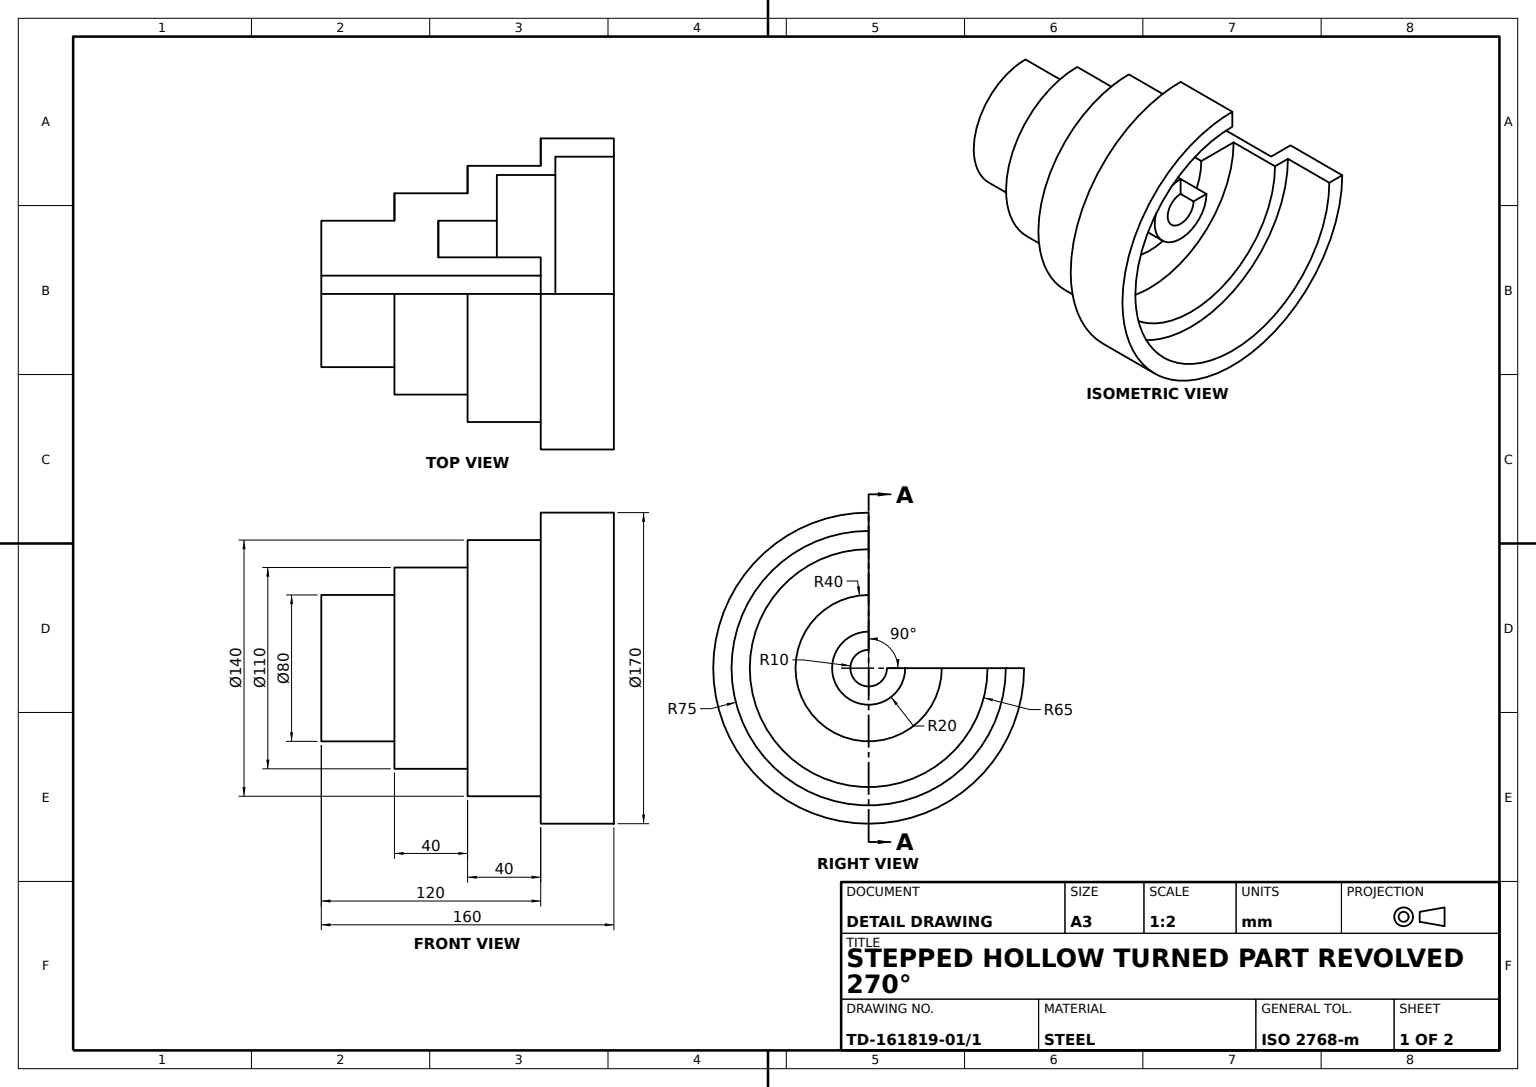
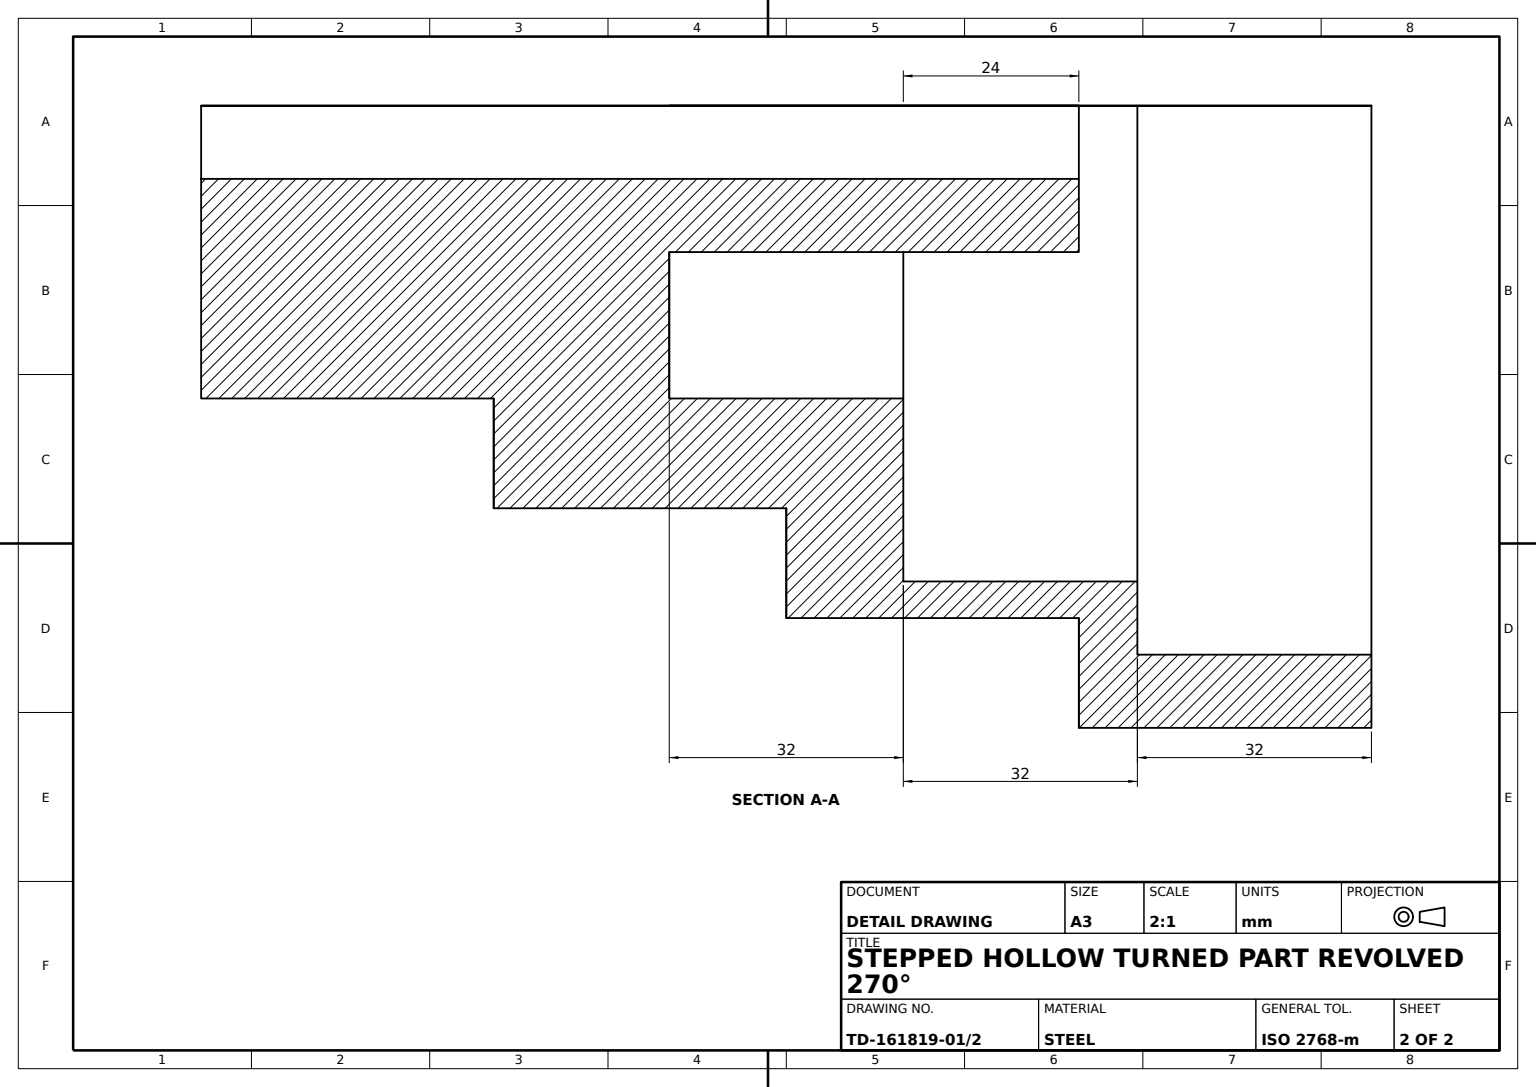
from build123d import *

# Parameters (mm, degrees)
HOUSING_REVOLVE_270DEG_ANGLE = 270


with BuildPart() as part:
    # Stepped Housing Profile → Housing Revolve 270deg (revolve)
    with BuildSketch(Plane.XY):
        Polygon((0, 40), (0, 10), (120, 10), (120, 20), (64, 20), (64, 40), (96, 40), (96, 65), (128, 65), (128, 75), (160, 75), (160, 85), (120, 85), (120, 70), (80, 70), (80, 55), (40, 55), (40, 40), align=None)
    revolve(axis=Axis((0, 0, 0), (1, 0, 0)), revolution_arc=HOUSING_REVOLVE_270DEG_ANGLE)


solid = part.part
